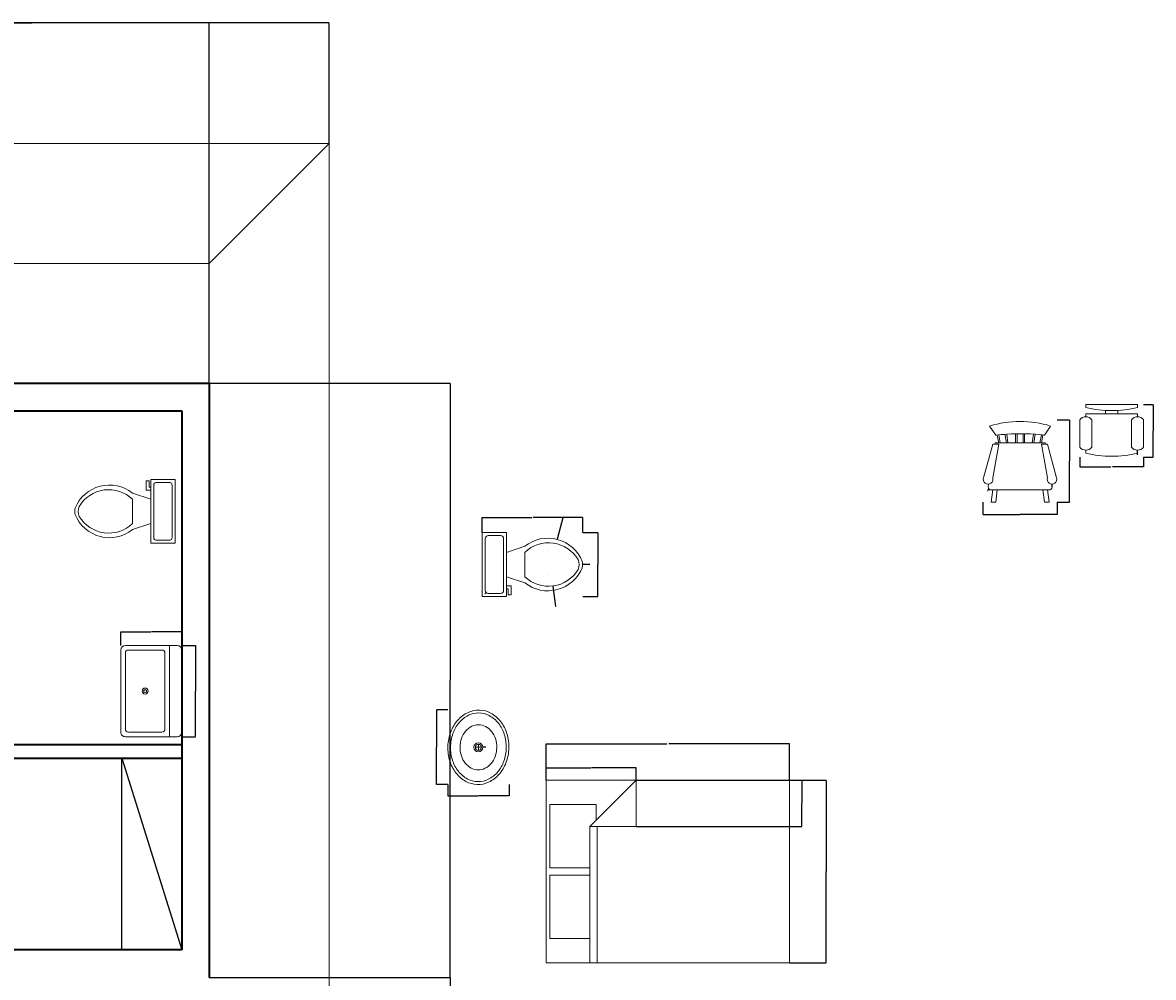
# Model space of a CAD drawing. Units: millimetres. Extents: x -8052 to 19968, y -37825 to -17505.
# Tile 10 of 10: x 10533 to 19968, y -25475 to -17505. Entities that reach past the tile are written whole.
import ezdxf

# ---------------------------------------------------------------- set-up
doc = ezdxf.new("R2010")
doc.units = ezdxf.units.MM
doc.header["$MEASUREMENT"] = 0
for name, color, linetype, lineweight in [('A-ANNO-DIMS', 2, 'Continuous', 18), ('A-FLOR', 8, 'Continuous', 18), ('A-FLOR-CASE', 9, 'Continuous', 25), ('A-FLOR-FIXT', 9, 'Continuous', 18), ('A-FURN', 8, 'Continuous', 18), ('A-WALL', 7, 'Continuous', 35)]:
    doc.layers.add(name, color=color, linetype=linetype, lineweight=lineweight)
doc.styles.get("Standard").update_dxf_attribs({"font": 'arial.ttf'})
doc.dimstyles.get("Standard").update_dxf_attribs({"dimtxt": 1.054, "dimasz": 1.055, "dimexe": 0.18, "dimexo": 0.0625, "dimgap": 0.09, "dimtad": 0, "dimtih": 1, "dimtoh": 1, "dimdec": 4, "dimzin": 0, "dimdsep": 46, "dimtxsty": 'Standard', "dimcen": 0.09, "dimadec": 0, "dimazin": 0, "dimtfac": 1, "dimtdec": 4, "dimtofl": 0, "dimtmove": 0, "dimatfit": 3, "dimfxl": 1, "dimtolj": 1, "dimtzin": 0, "dimarcsym": 0})

# ---------------------------------------------------------------- blocks, each defined once
blk = doc.blocks.new('Chair - Desk')
for p, q in [((-8.5, 0), (-8.5, -1)), ((-8.5, 0), (8.5, 0)), ((8.5, 0), (8.5, -1)), ((-8.5, -3), (-8.5, -4)), ((-8.5, -3), (8.5, -3)), ((-2, -3), (-2, -1.9355)), ((2, -1.9576), (2, -3)), ((8.5, -3), (8.5, -4)), ((-10.5, -5), (-10.5, -14)), ((-6.5, -14), (-6.5, -5)), ((6.5, -5), (6.5, -14)), ((10.5, -14), (10.5, -5)), ((-8.5, -15), (-8.5, -16)), ((8.5, -15), (8.5, -16))]:
    blk.add_line(p, q)
for centre, radius, start, end in [((0, 34.625), 36.625, 256.5803, 283.4197), ((-8.5, -6.5), 2.5, 36.8699, 143.1301), ((8.5, -6.5), 2.5, 36.8699, 143.1301), ((-8.5, -12.5), 2.5, 216.8699, 323.1301), ((8.5, -12.5), 2.5, 216.8699, 323.1301), ((0, 19.625), 36.625, 256.5803, 283.4197)]:
    blk.add_arc(centre, radius, start, end)
blk = doc.blocks.new('Chair - Rocking')
for p, q in [((-8, -4.5), (-10, -1.5)), ((8, -4.5), (10, -1.5)), ((-8.23428, -6.99939), (-8.3093, -7.47958)), ((-8.23041, -7), (8.23915, -7)), ((-7.5, -4.5), (-7, -7)), ((-6.5, -7), (-7.02225, -4.43)), ((-4.5, -7), (-4.96674, -4.19951)), ((-4, -7), (-4.40532, -4.16272)), ((-1.5, -4.05012), (-1.5, -7)), ((-1, -7), (-1, -4.05012)), ((1, -7), (1, -4.04655)), ((1.5, -4.05012), (1.5, -7)), ((4, -7), (4.40187, -4.18694)), ((4.5, -7), (4.96761, -4.19437)), ((6.5, -7), (7, -4.4057)), ((7.5, -4.5), (7, -7)), ((8.31071, -7.48854), (8.23449, -7.00073)), ((-9, -7.5), (-12, -18.49999)), ((-7, -7.5), (-9, -7.5)), ((-9, -18.49999), (-7, -7.5)), ((7, -7.5), (9, -7.5)), ((9, -18.49999), (7, -7.5)), ((9, -7.5), (12, -18.49999)), ((-10.36644, -20.64523), (-10.5, -21.49999)), ((10.5, -21.49999), (10.3575, -20.58798)), ((-9, -22.49999), (-9.5, -26.49999)), ((0, -22.49999), (-9.5, -22.49999)), ((-8, -26.49999), (-7.5, -22.49999)), ((0, -22.49999), (9.5, -22.49999)), ((8, -26.49999), (7.5, -22.49999)), ((9, -22.49999), (9.5, -26.49999)), ((-9.5, -26.49999), (-8, -26.49999)), ((9.5, -26.49999), (8, -26.49999))]:
    blk.add_line(p, q)
for centre, radius, start, end in [((0, -34.08333), 34.08333, 72.93847, 107.0615), ((0, -68.25004), 64.25, 93.92211, 97.15267), ((0, -68.25004), 64.25, 82.84733, 93.92211), ((-10.5, -18.99999), 1.58114, 161.5651, 18.43495), ((10.5, -18.99999), 1.58114, 161.5651, 18.43495), ((-9.5, -21.49999), 1, 180, 270), ((9.5, -21.49999), 1, 270, 0)]:
    blk.add_arc(centre, radius, start, end)
blk = doc.blocks.new('Toilet - top')
for p, q in [((9.5, -6), (9.5, -2)), ((-10, -8.5), (-8, -8.5)), ((-10, -9.5), (-10, -8.5)), ((-7, -9.5), (-10, -9.5)), ((-8, -8.5), (-8, -8)), ((-7, -8), (-7, -9.5)), ((-4, -8), (-6, -14)), ((4, -8), (6, -14)), ((4, -14), (-4, -14))]:
    blk.add_line(p, q)
blk.add_lwpolyline([(10.5, -8), (10.5, 0), (-10.5, 0), (-10.5, -8)], close=True)
for points in [[(-9.5, -2), (-9.5, -6)], [(8.5, -1), (-8.5, -1)], [(-8.5, -7), (8.5, -7)]]:
    blk.add_lwpolyline(points)
for centre, radius, start, end in [((-8.62, -1.88), 0.884, 81.8699, 188.1301), ((8.62, -1.88), 0.884, 351.8699, 98.1301), ((-8.62, -6.12), 0.884, 171.8699, 278.1301), ((8.62, -6.12), 0.884, 261.8699, 8.1301), ((3.52, -21.58), 12.17, 141.4691, 247.9714), ((4.2, -21.82), 11.33, 136.3677, 238.9468), ((-3.52, -21.58), 12.17, 292.0284, 38.5307), ((-4.2, -21.82), 11.33, 301.053, 43.6321), ((0, -27.88), 4, 245.7318, 294.2682), ((0, -29), 4, 254.8605, 285.1395)]:
    blk.add_arc(centre, radius, start, end)
blk = doc.blocks.new('Sink - Oval top')
for p, q in [((-1, 0), (1, 0)), ((0, 1), (0, -1))]:
    blk.add_line(p, q)
for points in [[(-12.23, 0.39, 0.117634), (-11.46, -3.36, 0.104469), (-8.88, -6.8, 0.090016), (-5.08, -9.07, 0.08192), (-0.32, -10.02, 0.08192), (4.49, -9.38, 0.090016), (8.42, -7.36, 0.104469), (11.22, -4.09, 0.117634), (12.23, -0.39, 0.117634), (11.46, 3.36, 0.104469), (8.88, 6.8, 0.090016), (5.08, 9.07, 0.08192), (0.32, 10.02, 0.08192), (-4.49, 9.38, 0.090016), (-8.42, 7.36, 0.104469), (-11.22, 4.09, 0.117634)], [(-11.29, 0.16, 0.118622), (-10.52, -3.25, 0.104678), (-8.07, -6.36, 0.089562), (-4.54, -8.37, 0.081185), (-0.13, -9.15, 0.081185), (4.3, -8.49, 0.089562), (7.89, -6.58, 0.104678), (10.42, -3.55, 0.118622), (11.29, -0.16, 0.118622), (10.52, 3.25, 0.104678), (8.07, 6.36, 0.089562), (4.54, 8.37, 0.081185), (0.13, 9.15, 0.081185), (-4.3, 8.49, 0.089562), (-7.89, 6.58, 0.104678), (-10.42, 3.55, 0.118622)], [(-7.42, 0.08, 0.118283), (-6.91, -2.17, 0.104607), (-5.29, -4.21, 0.089718), (-2.97, -5.53, 0.081436), (-0.07, -6.04, 0.081436), (2.84, -5.59, 0.089718), (5.2, -4.33, 0.104607), (6.86, -2.32, 0.118283), (7.42, -0.08, 0.118283), (6.91, 2.17, 0.104607), (5.29, 4.21, 0.089718), (2.97, 5.53, 0.081436), (0.07, 6.04, 0.081436), (-2.84, 5.59, 0.089718), (-5.2, 4.33, 0.104607), (-6.86, 2.32, 0.118283)]]:
    blk.add_lwpolyline(points, format="xyb", close=True)
for radius in [1.5, 1]:
    blk.add_circle((0, 0), radius)
blk = doc.blocks.new('Bed - Queen')
for p, q in [((0, -80.00003), (0, 0)), ((0, 0), (59.99999, 0)), ((59.99999, 0), (59.99999, -80.00003)), ((7.99999, -1.2), (28.79998, -1.2)), ((7.99999, -14.4), (7.99999, -1.2)), ((28.79998, -1.2), (28.79998, -14.4)), ((31.19999, -1.2), (51.99999, -1.2)), ((31.19999, -14.4), (31.19999, -1.2)), ((51.99999, -1.2), (51.99999, -16.4)), ((0, -14.4), (44.8, -14.4)), ((59.99999, -29.6), (44.8, -14.4)), ((44.8, -14.4), (44.8, -29.6)), ((44.8, -16.8), (0, -16.8)), ((51.99999, -16.4), (46.79936, -16.4)), ((44.8, -29.6), (59.99999, -29.6)), ((59.99999, -80.00003), (0, -80.00003))]:
    blk.add_line(p, q)
blk = doc.blocks.new('Sink-single - 30 in top')
blk.add_line((-15, -3.999996), (15, -3.999996))
for points in [[(-13.5, 0), (13.5, 0)], [(-15, -18.499996), (-15, -1.5)], [(15, -1.5), (15, -18.499996)], [(-13.5, -17.499996), (-13.5, -6.499996)], [(-12.5, -5.499996), (12.5, -5.499996)], [(13.5, -6.499996), (13.5, -17.499996)], [(12.5, -18.499996), (-12.5, -18.499996)], [(13.5, -19.999996), (-13.5, -19.999996)]]:
    blk.add_lwpolyline(points)
for radius in [1, 0.5]:
    blk.add_circle((0, -11.999996), radius)
for centre, radius, start, end in [((-13.5, -1.5), 1.5, 90, 180), ((13.5, -1.5), 1.5, 0, 90), ((-12.5, -6.499996), 1, 90, 180), ((12.5, -6.499996), 1, 0, 90), ((-13.5, -18.499996), 1.5, 180, 270), ((-12.5, -17.499996), 1, 180, 270), ((12.5, -17.499996), 1, 270, 0), ((13.5, -18.499996), 1.5, 270, 0)]:
    blk.add_arc(centre, radius, start, end)
blk = doc.blocks.new('CABINET-RECESSED-1600')
for p, q in [((500, 1600), (0, 0)), ((500, 0), (500, 1600))]:
    blk.add_line(p, q)
blk = doc.blocks.new('*D34')
at = {"layer": 'A-ANNO-DIMS', "color": 0, "lineweight": -2, "transparency": 16777216}
for p, q in [((14901.3, -23828.8), (14901.3, -23523.9)), ((14902.3, -23524.1), (15909.3, -23524.1)), ((16932.2, -23524.1), (15925.3, -23524.1)), ((16933.3, -23828.8), (16933.3, -23523.9))]:
    blk.add_line(p, q, dxfattribs=at)
at = {"layer": 'A-ANNO-DIMS', "color": 0, "lineweight": 100, "transparency": 16777216}
for points in [[(14902.3, -23523.9), (14902.3, -23524.2), (14901.3, -23524.1)], [(16932.2, -23523.9), (16932.2, -23524.2), (16933.3, -23524.1)]]:
    blk.add_solid(points, dxfattribs=at)
at = {"layer": 'Defpoints', "color": 0, "lineweight": 100, "transparency": 16777216}
for p in [(14901.3, -23524.1), (14901.3, -23828.9), (16933.3, -23828.9)]:
    blk.add_point(p, dxfattribs=at)
at = {"layer": 'A-ANNO-DIMS', "color": 0, "transparency": 16777216, "insert": (15917.3, -23524.1), "char_height": 1.054, "attachment_point": 5}
blk.add_mtext('\\A1;QUEEN BED 2032 TYP.', dxfattribs=at)
blk = doc.blocks.new('*D35')
at = {"layer": 'A-ANNO-DIMS', "color": 0, "lineweight": -2, "transparency": 16777216}
for p, q in [((16933.3, -23828.9), (17238.3, -23828.9)), ((17238.1, -23829.9), (17238.1, -24590.2)), ((17238.1, -25351.8), (17238.1, -24591.5)), ((16933.3, -25352.9), (17238.3, -25352.9))]:
    blk.add_line(p, q, dxfattribs=at)
at = {"layer": 'A-ANNO-DIMS', "color": 0, "lineweight": 100, "transparency": 16777216}
for points in [[(17237.9, -23829.9), (17238.2, -23829.9), (17238.1, -23828.9)], [(17237.9, -25351.8), (17238.2, -25351.8), (17238.1, -25352.9)]]:
    blk.add_solid(points, dxfattribs=at)
at = {"layer": 'Defpoints', "color": 0, "lineweight": 100, "transparency": 16777216}
for p in [(16933.3, -23828.9), (17238.1, -23828.9), (16933.3, -25352.9)]:
    blk.add_point(p, dxfattribs=at)
at = {"layer": 'A-ANNO-DIMS', "color": 0, "transparency": 16777216, "insert": (17238.1, -24590.9), "char_height": 1.054, "attachment_point": 5}
blk.add_mtext('\\A1;1524 TYP.', dxfattribs=at)
blk = doc.blocks.new('*D36')
at = {"layer": 'A-ANNO-DIMS', "color": 0, "lineweight": -2, "transparency": 16777216}
for p, q in [((14367.7, -21761.6), (14367.7, -21635.5)), ((14368.7, -21635.7), (14782.8, -21635.7)), ((15206, -21635.7), (14791.9, -21635.7)), ((15207, -21761.6), (15207, -21635.5))]:
    blk.add_line(p, q, dxfattribs=at)
at = {"layer": 'A-ANNO-DIMS', "color": 0, "lineweight": 100, "transparency": 16777216}
for points in [[(14368.7, -21635.6), (14368.7, -21635.9), (14367.7, -21635.7)], [(15206, -21635.6), (15206, -21635.9), (15207, -21635.7)]]:
    blk.add_solid(points, dxfattribs=at)
at = {"layer": 'Defpoints', "color": 0, "lineweight": 100, "transparency": 16777216}
for p in [(14367.7, -21635.7), (14367.7, -21761.6), (15207, -21761.6)]:
    blk.add_point(p, dxfattribs=at)
at = {"layer": 'A-ANNO-DIMS', "color": 0, "transparency": 16777216, "insert": (14787.3, -21635.7), "char_height": 1.054, "attachment_point": 5}
blk.add_mtext('\\A1;WC 839 TYP.', dxfattribs=at)
blk = doc.blocks.new('*D37')
at = {"layer": 'A-ANNO-DIMS', "color": 0, "lineweight": -2, "transparency": 16777216}
for p, q in [((15207.1, -21761.6), (15333.1, -21761.6)), ((15332.9, -21762.7), (15332.9, -22027.7)), ((15332.9, -22294), (15332.9, -22029)), ((15207.1, -22295), (15333.1, -22295))]:
    blk.add_line(p, q, dxfattribs=at)
at = {"layer": 'A-ANNO-DIMS', "color": 0, "lineweight": 100, "transparency": 16777216}
for points in [[(15332.8, -21762.7), (15333.1, -21762.7), (15332.9, -21761.6)], [(15332.8, -22294), (15333.1, -22294), (15332.9, -22295)]]:
    blk.add_solid(points, dxfattribs=at)
at = {"layer": 'Defpoints', "color": 0, "lineweight": 100, "transparency": 16777216}
for p in [(15207, -21761.6), (15332.9, -21761.6), (15207, -22295)]:
    blk.add_point(p, dxfattribs=at)
at = {"layer": 'A-ANNO-DIMS', "color": 0, "transparency": 16777216, "insert": (15332.9, -22028.3), "char_height": 1.054, "attachment_point": 5}
blk.add_mtext('\\A1;533 TYP.', dxfattribs=at)
blk = doc.blocks.new('*D38')
at = {"layer": 'A-ANNO-DIMS', "color": 0, "lineweight": -2, "transparency": 16777216}
for p, q in [((14080.1, -23242.4), (13986.4, -23242.4)), ((13986.6, -23243.4), (13986.6, -23553.5)), ((13986.6, -23864.9), (13986.6, -23554.8)), ((14080.1, -23865.9), (13986.4, -23865.9))]:
    blk.add_line(p, q, dxfattribs=at)
at = {"layer": 'A-ANNO-DIMS', "color": 0, "lineweight": 100, "transparency": 16777216}
for points in [[(13986.4, -23243.4), (13986.8, -23243.4), (13986.6, -23242.4)], [(13986.4, -23864.9), (13986.8, -23864.9), (13986.6, -23865.9)]]:
    blk.add_solid(points, dxfattribs=at)
at = {"layer": 'Defpoints', "color": 0, "lineweight": 100, "transparency": 16777216}
for p in [(14080.1, -23242.4), (13986.6, -23865.9), (14080.1, -23865.9)]:
    blk.add_point(p, dxfattribs=at)
at = {"layer": 'A-ANNO-DIMS', "color": 0, "transparency": 16777216, "insert": (13986.6, -23554.2), "char_height": 1.054, "attachment_point": 5}
blk.add_mtext('\\A1;BASIN 624 TYP.', dxfattribs=at)
blk = doc.blocks.new('*D39')
at = {"layer": 'A-ANNO-DIMS', "color": 0, "lineweight": -2, "transparency": 16777216}
for p, q in [((14080.1, -23866), (14080.1, -23959.7)), ((14591.6, -23866), (14591.6, -23959.7)), ((14081.2, -23959.5), (14332.8, -23959.5)), ((14590.5, -23959.5), (14338.9, -23959.5))]:
    blk.add_line(p, q, dxfattribs=at)
at = {"layer": 'A-ANNO-DIMS', "color": 0, "lineweight": 100, "transparency": 16777216}
for points in [[(14081.2, -23959.3), (14081.2, -23959.7), (14080.1, -23959.5)], [(14590.5, -23959.3), (14590.5, -23959.7), (14591.6, -23959.5)]]:
    blk.add_solid(points, dxfattribs=at)
at = {"layer": 'Defpoints', "color": 0, "lineweight": 100, "transparency": 16777216}
for p in [(14080.1, -23865.9), (14591.6, -23865.9), (14591.6, -23959.5)]:
    blk.add_point(p, dxfattribs=at)
at = {"layer": 'A-ANNO-DIMS', "color": 0, "transparency": 16777216, "insert": (14335.9, -23959.5), "char_height": 1.054, "attachment_point": 5}
blk.add_mtext('\\A1;511 TYP.', dxfattribs=at)
blk = doc.blocks.new('*D40')
at = {"layer": 'A-ANNO-DIMS', "color": 0, "lineweight": -2, "transparency": 16777216}
for p, q in [((19353.6, -21133.4), (19353.6, -21213.5)), ((19887, -21133.4), (19887, -21213.5)), ((19354.7, -21213.3), (19614.4, -21213.3)), ((19886, -21213.3), (19626.3, -21213.3))]:
    blk.add_line(p, q, dxfattribs=at)
at = {"layer": 'A-ANNO-DIMS', "color": 0, "lineweight": 100, "transparency": 16777216}
for points in [[(19354.7, -21213.1), (19354.7, -21213.5), (19353.6, -21213.3)], [(19886, -21213.1), (19886, -21213.5), (19887, -21213.3)]]:
    blk.add_solid(points, dxfattribs=at)
at = {"layer": 'Defpoints', "color": 0, "lineweight": 100, "transparency": 16777216}
for p in [(19353.6, -21133.3), (19887, -21133.3), (19887, -21213.3)]:
    blk.add_point(p, dxfattribs=at)
at = {"layer": 'A-ANNO-DIMS', "color": 0, "transparency": 16777216, "insert": (19620.3, -21213.3), "char_height": 1.054, "attachment_point": 5}
blk.add_mtext('\\A1;DESK CHAIR 533', dxfattribs=at)
blk = doc.blocks.new('*D41')
at = {"layer": 'A-ANNO-DIMS', "color": 0, "lineweight": -2, "transparency": 16777216}
for p, q in [((19887.1, -20693), (19967.2, -20693)), ((19967, -20694.1), (19967, -20912.5)), ((19967, -21132.2), (19967, -20913.8)), ((19887.1, -21133.3), (19967.2, -21133.3))]:
    blk.add_line(p, q, dxfattribs=at)
at = {"layer": 'A-ANNO-DIMS', "color": 0, "lineweight": 100, "transparency": 16777216}
for points in [[(19966.9, -20694.1), (19967.2, -20694.1), (19967, -20693)], [(19966.9, -21132.2), (19967.2, -21132.2), (19967, -21133.3)]]:
    blk.add_solid(points, dxfattribs=at)
at = {"layer": 'Defpoints', "color": 0, "lineweight": 100, "transparency": 16777216}
for p in [(19887, -20693), (19967, -20693), (19887, -21133.3)]:
    blk.add_point(p, dxfattribs=at)
at = {"layer": 'A-ANNO-DIMS', "color": 0, "transparency": 16777216, "insert": (19967, -20913.2), "char_height": 1.05, "attachment_point": 5}
blk.add_mtext('\\A1;440', dxfattribs=at)
blk = doc.blocks.new('*D42')
at = {"layer": 'A-ANNO-DIMS', "color": 0, "lineweight": -2, "transparency": 16777216}
for p, q in [((19166.6, -20821.7), (19269.6, -20821.7)), ((19269.4, -20822.8), (19269.4, -21164)), ((19269.4, -21506.5), (19269.4, -21165.3)), ((19166.6, -21507.5), (19269.6, -21507.5))]:
    blk.add_line(p, q, dxfattribs=at)
at = {"layer": 'A-ANNO-DIMS', "color": 0, "lineweight": 100, "transparency": 16777216}
for points in [[(19269.2, -20822.8), (19269.6, -20822.8), (19269.4, -20821.7)], [(19269.2, -21506.5), (19269.6, -21506.5), (19269.4, -21507.5)]]:
    blk.add_solid(points, dxfattribs=at)
at = {"layer": 'Defpoints', "color": 0, "lineweight": 100, "transparency": 16777216}
for p in [(19166.5, -20821.7), (19269.4, -20821.7), (19166.5, -21507.5)]:
    blk.add_point(p, dxfattribs=at)
at = {"layer": 'A-ANNO-DIMS', "color": 0, "transparency": 16777216, "insert": (19269.4, -21164.6), "char_height": 1.054, "attachment_point": 5}
blk.add_mtext('\\A1;ROCKER 686', dxfattribs=at)
blk = doc.blocks.new('*D43')
at = {"layer": 'A-ANNO-DIMS', "color": 0, "lineweight": -2, "transparency": 16777216}
for p, q in [((18545.9, -21507.6), (18545.9, -21610.6)), ((19166.5, -21507.6), (19166.5, -21610.6)), ((18546.9, -21610.4), (18855.1, -21610.4)), ((19165.5, -21610.4), (18857.4, -21610.4))]:
    blk.add_line(p, q, dxfattribs=at)
at = {"layer": 'A-ANNO-DIMS', "color": 0, "lineweight": 100, "transparency": 16777216}
for points in [[(18546.9, -21610.2), (18546.9, -21610.6), (18545.9, -21610.4)], [(19165.5, -21610.2), (19165.5, -21610.6), (19166.5, -21610.4)]]:
    blk.add_solid(points, dxfattribs=at)
at = {"layer": 'Defpoints', "color": 0, "lineweight": 100, "transparency": 16777216}
for p in [(18545.9, -21507.5), (19166.5, -21507.5), (19166.5, -21610.4)]:
    blk.add_point(p, dxfattribs=at)
at = {"layer": 'A-ANNO-DIMS', "color": 0, "transparency": 16777216, "insert": (18856.2, -21610.4), "char_height": 1.05, "attachment_point": 5}
blk.add_mtext('\\A1;621', dxfattribs=at)
blk = doc.blocks.new('*D44')
at = {"layer": 'A-ANNO-DIMS', "color": 0, "lineweight": -2, "transparency": 16777216}
for p, q in [((11860, -22703.8), (11974.5, -22703.8)), ((11974.3, -22704.9), (11974.3, -23084.2)), ((11974.3, -23464.7), (11974.3, -23085.4)), ((11860, -23465.8), (11974.5, -23465.8))]:
    blk.add_line(p, q, dxfattribs=at)
at = {"layer": 'A-ANNO-DIMS', "color": 0, "lineweight": 100, "transparency": 16777216}
for points in [[(11974.1, -22704.9), (11974.5, -22704.9), (11974.3, -22703.8)], [(11974.1, -23464.7), (11974.5, -23464.7), (11974.3, -23465.8)]]:
    blk.add_solid(points, dxfattribs=at)
at = {"layer": 'Defpoints', "color": 0, "lineweight": 100, "transparency": 16777216}
for p in [(11860, -22703.8), (11860, -23465.8), (11974.3, -23465.8)]:
    blk.add_point(p, dxfattribs=at)
at = {"layer": 'A-ANNO-DIMS', "color": 0, "transparency": 16777216, "insert": (11974.3, -23084.8), "char_height": 1.054, "attachment_point": 5}
blk.add_mtext('\\A1;VANITY SINK 762 TYP.', dxfattribs=at)
blk = doc.blocks.new('*D45')
at = {"layer": 'A-ANNO-DIMS', "color": 0, "lineweight": -2, "transparency": 16777216}
for p, q in [((11352, -22703.7), (11352, -22589.3)), ((11353, -22589.5), (11602.9, -22589.5)), ((11858.9, -22589.5), (11609, -22589.5)), ((11860, -22703.7), (11860, -22589.3))]:
    blk.add_line(p, q, dxfattribs=at)
at = {"layer": 'A-ANNO-DIMS', "color": 0, "lineweight": 100, "transparency": 16777216}
for points in [[(11353, -22589.3), (11353, -22589.7), (11352, -22589.5)], [(11858.9, -22589.3), (11858.9, -22589.7), (11860, -22589.5)]]:
    blk.add_solid(points, dxfattribs=at)
at = {"layer": 'Defpoints', "color": 0, "lineweight": 100, "transparency": 16777216}
for p in [(11860, -22589.5), (11352, -22703.8), (11860, -22703.8)]:
    blk.add_point(p, dxfattribs=at)
at = {"layer": 'A-ANNO-DIMS', "color": 0, "transparency": 16777216, "insert": (11606, -22589.5), "char_height": 1.054, "attachment_point": 5}
blk.add_mtext('\\A1;508 TYP.', dxfattribs=at)
blk = doc.blocks.new('*D84')
at = {"layer": 'A-ANNO-DIMS', "color": 0, "lineweight": -2, "transparency": 16777216}
for p, q in [((-7040, -18514.8), (-7040, -17505.2)), ((-7039, -17505.3), (3022.9, -17505.3)), ((13088.9, -17505.3), (3027.1, -17505.3)), ((13090, -18514.8), (13090, -17505.2))]:
    blk.add_line(p, q, dxfattribs=at)
at = {"layer": 'A-ANNO-DIMS', "color": 0, "lineweight": 100, "transparency": 16777216}
for points in [[(-7039, -17505.2), (-7039, -17505.5), (-7040, -17505.3)], [(13088.9, -17505.2), (13088.9, -17505.5), (13090, -17505.3)]]:
    blk.add_solid(points, dxfattribs=at)
at = {"layer": 'Defpoints', "color": 0, "lineweight": 100, "transparency": 16777216}
for p in [(13090, -17505.3), (-7040, -18514.8), (13090, -18514.8)]:
    blk.add_point(p, dxfattribs=at)
at = {"layer": 'A-ANNO-DIMS', "color": 0, "transparency": 16777216, "insert": (3025, -17505.3), "char_height": 1.05, "attachment_point": 5}
blk.add_mtext('\\A1;20130', dxfattribs=at)
blk = doc.blocks.new('*D93')
at = {"layer": 'A-ANNO-DIMS', "color": 0, "lineweight": -2, "transparency": 16777216}
for p, q in [((9130, -20514.8), (9130, -17505.2)), ((9131, -17505.3), (10608.3, -17505.3)), ((12088.9, -17505.3), (10611.7, -17505.3)), ((12090, -20514.8), (12090, -17505.2))]:
    blk.add_line(p, q, dxfattribs=at)
at = {"layer": 'A-ANNO-DIMS', "color": 0, "lineweight": 100, "transparency": 16777216}
for points in [[(9131, -17505.2), (9131, -17505.5), (9130, -17505.3)], [(12088.9, -17505.2), (12088.9, -17505.5), (12090, -17505.3)]]:
    blk.add_solid(points, dxfattribs=at)
at = {"layer": 'Defpoints', "color": 0, "lineweight": 100, "transparency": 16777216}
for p in [(12090, -17505.3), (9130, -20514.8), (12090, -20514.8)]:
    blk.add_point(p, dxfattribs=at)
at = {"layer": 'A-ANNO-DIMS', "color": 0, "transparency": 16777216, "insert": (10610, -17505.3), "char_height": 1.05, "attachment_point": 5}
blk.add_mtext('\\A1;2960', dxfattribs=at)
blk = doc.blocks.new('*D96')
at = {"layer": 'A-ANNO-DIMS', "color": 0, "lineweight": -2, "transparency": 16777216}
for p, q in [((12090, -20514.8), (14099.7, -20514.8)), ((14099.5, -20515.9), (14099.5, -22994.2)), ((14099.5, -25473.8), (14099.5, -22995.5)), ((12090, -25474.8), (14099.7, -25474.8))]:
    blk.add_line(p, q, dxfattribs=at)
at = {"layer": 'A-ANNO-DIMS', "color": 0, "lineweight": 100, "transparency": 16777216}
for points in [[(14099.3, -20515.9), (14099.7, -20515.9), (14099.5, -20514.8)], [(14099.3, -25473.8), (14099.7, -25473.8), (14099.5, -25474.8)]]:
    blk.add_solid(points, dxfattribs=at)
at = {"layer": 'Defpoints', "color": 0, "lineweight": 100, "transparency": 16777216}
for p in [(12090, -20514.8), (12090, -25474.8), (14099.5, -25474.8)]:
    blk.add_point(p, dxfattribs=at)
at = {"layer": 'A-ANNO-DIMS', "color": 0, "transparency": 16777216, "insert": (14099.5, -22994.8), "char_height": 1.05, "attachment_point": 5}
blk.add_mtext('\\A1;4960', dxfattribs=at)
blk = doc.blocks.new('*D97')
at = {"layer": 'A-ANNO-DIMS', "color": 0, "lineweight": -2, "transparency": 16777216}
for p, q in [((12090, -25474.8), (14099.7, -25474.8)), ((14099.5, -25475.9), (14099.5, -27724.2)), ((14099.5, -29973.8), (14099.5, -27725.5)), ((10410, -29974.8), (14099.7, -29974.8))]:
    blk.add_line(p, q, dxfattribs=at)
at = {"layer": 'A-ANNO-DIMS', "color": 0, "lineweight": 100, "transparency": 16777216}
for points in [[(14099.3, -25475.9), (14099.7, -25475.9), (14099.5, -25474.8)], [(14099.3, -29973.8), (14099.7, -29973.8), (14099.5, -29974.8)]]:
    blk.add_solid(points, dxfattribs=at)
at = {"layer": 'Defpoints', "color": 0, "lineweight": 100, "transparency": 16777216}
for p in [(12090, -25474.8), (10410, -29974.8), (14099.5, -29974.8)]:
    blk.add_point(p, dxfattribs=at)
at = {"layer": 'A-ANNO-DIMS', "color": 0, "transparency": 16777216, "insert": (14099.5, -27724.8), "char_height": 1.05, "attachment_point": 5}
blk.add_mtext('\\A1;4500', dxfattribs=at)
blk = doc.blocks.new('*D123')
at = {"layer": 'A-ANNO-DIMS', "color": 0, "lineweight": -2, "transparency": 16777216}
for p, q in [((7260, -25474.8), (7260, -17505.2)), ((7261, -17505.3), (9673.3, -17505.3)), ((12088.9, -17505.3), (9676.7, -17505.3)), ((12090, -25474.8), (12090, -17505.2))]:
    blk.add_line(p, q, dxfattribs=at)
at = {"layer": 'A-ANNO-DIMS', "color": 0, "lineweight": 100, "transparency": 16777216}
for points in [[(7261, -17505.2), (7261, -17505.5), (7260, -17505.3)], [(12088.9, -17505.2), (12088.9, -17505.5), (12090, -17505.3)]]:
    blk.add_solid(points, dxfattribs=at)
at = {"layer": 'Defpoints', "color": 0, "lineweight": 100, "transparency": 16777216}
for p in [(7260, -17505.3), (7260, -25474.8), (12090, -25474.8)]:
    blk.add_point(p, dxfattribs=at)
at = {"layer": 'A-ANNO-DIMS', "color": 0, "transparency": 16777216, "insert": (9675, -17505.3), "char_height": 1.05, "attachment_point": 5}
blk.add_mtext('\\A1;4830', dxfattribs=at)
blk = doc.blocks.new('*D129')
at = {"layer": 'A-ANNO-DIMS', "color": 0, "lineweight": -2, "transparency": 16777216}
for p, q in [((14901.3, -23828.8), (14901.3, -23725.9)), ((14902.3, -23726.1), (15275.3, -23726.1)), ((15652.1, -23726.1), (15279.1, -23726.1)), ((15653.1, -23828.8), (15653.1, -23725.9))]:
    blk.add_line(p, q, dxfattribs=at)
at = {"layer": 'A-ANNO-DIMS', "color": 0, "lineweight": 100, "transparency": 16777216}
for points in [[(14902.3, -23725.9), (14902.3, -23726.3), (14901.3, -23726.1)], [(15652.1, -23725.9), (15652.1, -23726.3), (15653.1, -23726.1)]]:
    blk.add_solid(points, dxfattribs=at)
at = {"layer": 'Defpoints', "color": 0, "lineweight": 100, "transparency": 16777216}
for p in [(15653.1, -23726.1), (14901.3, -23828.9), (15653.1, -23828.9)]:
    blk.add_point(p, dxfattribs=at)
at = {"layer": 'A-ANNO-DIMS', "color": 0, "transparency": 16777216, "insert": (15277.2, -23726.1), "char_height": 1.05, "attachment_point": 5}
blk.add_mtext('\\A1;751.8', dxfattribs=at)
blk = doc.blocks.new('*D130')
at = {"layer": 'A-ANNO-DIMS', "color": 0, "lineweight": -2, "transparency": 16777216}
for p, q in [((15653.2, -23828.9), (17036.2, -23828.9)), ((17036, -23829.9), (17036, -24021.3)), ((17036, -24213.9), (17036, -24022.5)), ((15653.2, -24214.9), (17036.2, -24214.9))]:
    blk.add_line(p, q, dxfattribs=at)
at = {"layer": 'A-ANNO-DIMS', "color": 0, "lineweight": 100, "transparency": 16777216}
for points in [[(17035.8, -23829.9), (17036.2, -23829.9), (17036, -23828.9)], [(17035.8, -24213.9), (17036.2, -24213.9), (17036, -24214.9)]]:
    blk.add_solid(points, dxfattribs=at)
at = {"layer": 'Defpoints', "color": 0, "lineweight": 100, "transparency": 16777216}
for p in [(15653.1, -23828.9), (15653.1, -24214.9), (17036, -24214.9)]:
    blk.add_point(p, dxfattribs=at)
at = {"layer": 'A-ANNO-DIMS', "color": 0, "transparency": 16777216, "insert": (17036, -24021.9), "char_height": 1.05, "attachment_point": 5}
blk.add_mtext('\\A1;386.1', dxfattribs=at)
blk = doc.blocks.new('*D137')
at = {"layer": 'A-ANNO-DIMS', "color": 0, "lineweight": -2, "transparency": 16777216}
for p, q in [((15041.5, -21639.4), (14994.6, -21817.8)), ((15042.5, -21639.4), (15041.5, -21639.4)), ((14915.7, -22117.7), (14915.9, -22117.7)), ((14915.8, -22117.8), (14915.8, -22117.6))]:
    blk.add_line(p, q, dxfattribs=at)
at = {"layer": 'A-ANNO-DIMS', "color": 0, "lineweight": 100, "transparency": 16777216}
blk.add_solid([(14994.4, -21817.7), (14994.8, -21817.8), (14994.3, -21818.8)], dxfattribs=at)
at = {"layer": 'Defpoints', "color": 0, "lineweight": 100, "transparency": 16777216}
for p in [(14994.3, -21818.8), (14915.8, -22117.7)]:
    blk.add_point(p, dxfattribs=at)
at = {"layer": 'A-ANNO-DIMS', "color": 0, "transparency": 16777216, "insert": (15045.9, -21639.4), "char_height": 1.054, "attachment_point": 5}
blk.add_mtext('\\A1;2X R309.1', dxfattribs=at)
blk = doc.blocks.new('*D138')
at = {"layer": 'A-ANNO-DIMS', "color": 0, "lineweight": -2, "transparency": 16777216}
for p, q in [((14921.7, -21921.7), (14921.9, -21921.7)), ((14921.8, -21921.7), (14921.8, -21921.6)), ((14983.2, -22378), (14960.3, -22207.9)), ((14984.2, -22378), (14983.2, -22378))]:
    blk.add_line(p, q, dxfattribs=at)
at = {"layer": 'A-ANNO-DIMS', "color": 0, "lineweight": 100, "transparency": 16777216}
blk.add_solid([(14960.5, -22207.9), (14960.1, -22207.9), (14960.2, -22206.9)], dxfattribs=at)
at = {"layer": 'Defpoints', "color": 0, "lineweight": 100, "transparency": 16777216}
for p in [(14921.8, -21921.7), (14960.2, -22206.9)]:
    blk.add_point(p, dxfattribs=at)
at = {"layer": 'A-ANNO-DIMS', "color": 0, "transparency": 16777216, "insert": (14988.2, -22378), "char_height": 1.054, "attachment_point": 5}
blk.add_mtext('\\A1;2X R287.76', dxfattribs=at)
blk = doc.blocks.new('*D139')
at = {"layer": 'A-ANNO-DIMS', "color": 0, "lineweight": -2, "transparency": 16777216}
for p, q in [((15104.2, -22028.3), (15104.3, -22028.3)), ((15104.3, -22028.4), (15104.3, -22028.2)), ((15266.8, -22028.3), (15206.9, -22028.3))]:
    blk.add_line(p, q, dxfattribs=at)
at = {"layer": 'A-ANNO-DIMS', "color": 0, "lineweight": 100, "transparency": 16777216}
blk.add_solid([(15206.9, -22028.2), (15206.9, -22028.5), (15205.9, -22028.3)], dxfattribs=at)
at = {"layer": 'Defpoints', "color": 0, "lineweight": 100, "transparency": 16777216}
for p in [(15104.3, -22028.3), (15205.9, -22028.3)]:
    blk.add_point(p, dxfattribs=at)
at = {"layer": 'A-ANNO-DIMS', "color": 0, "transparency": 16777216, "insert": (15270.3, -22028.3), "char_height": 1.054, "attachment_point": 5}
blk.add_mtext('\\A1;2X R101.6', dxfattribs=at)
blk = doc.blocks.new('*D140')
at = {"layer": 'A-ANNO-DIMS', "color": 0, "lineweight": -2, "transparency": 16777216}
for p, q in [((14389.9, -22272.8), (14398.7, -22264)), ((14415.2, -22247.4), (14415.4, -22247.4)), ((14415.3, -22247.5), (14415.3, -22247.3)), ((14388.8, -22272.8), (14389.9, -22272.8))]:
    blk.add_line(p, q, dxfattribs=at)
at = {"layer": 'A-ANNO-DIMS', "color": 0, "lineweight": 100, "transparency": 16777216}
blk.add_solid([(14398.5, -22263.9), (14398.8, -22264.2), (14399.4, -22263.3)], dxfattribs=at)
at = {"layer": 'Defpoints', "color": 0, "lineweight": 100, "transparency": 16777216}
for p in [(14399.4, -22263.3), (14415.3, -22247.4)]:
    blk.add_point(p, dxfattribs=at)
at = {"layer": 'A-ANNO-DIMS', "color": 0, "transparency": 16777216, "insert": (14385.3, -22272.8), "char_height": 1.054, "attachment_point": 5}
blk.add_mtext('\\A1;4X R22.45', dxfattribs=at)
blk = doc.blocks.new('*D141')
at = {"layer": 'A-ANNO-DIMS', "color": 0, "lineweight": -2, "transparency": 16777216}
for p, q in [((14335.8, -23554.2), (14335.9, -23554.2)), ((14335.9, -23554.2), (14335.9, -23554.1)), ((14396.8, -23554.2), (14375, -23554.2))]:
    blk.add_line(p, q, dxfattribs=at)
at = {"layer": 'A-ANNO-DIMS', "color": 0, "lineweight": 100, "transparency": 16777216}
blk.add_solid([(14375, -23554), (14375, -23554.3), (14374, -23554.2)], dxfattribs=at)
at = {"layer": 'Defpoints', "color": 0, "lineweight": 100, "transparency": 16777216}
for p in [(14297.8, -23554.2), (14374, -23554.2)]:
    blk.add_point(p, dxfattribs=at)
at = {"layer": 'A-ANNO-DIMS', "color": 0, "transparency": 16777216, "insert": (14398.8, -23554.2), "char_height": 1.05, "attachment_point": 5}
blk.add_mtext('\\A1;∅76.2', dxfattribs=at)
blk = doc.blocks.new('*D142')
at = {"layer": 'A-ANNO-DIMS', "color": 0, "lineweight": -2, "transparency": 16777216}
for p, q in [((19122.8, -21317), (19123, -21317)), ((19122.9, -21317.1), (19122.9, -21317)), ((19122.9, -21381.3), (19122.9, -21358.3)), ((19124, -21381.3), (19122.9, -21381.3))]:
    blk.add_line(p, q, dxfattribs=at)
at = {"layer": 'A-ANNO-DIMS', "color": 0, "lineweight": 100, "transparency": 16777216}
blk.add_solid([(19123.1, -21358.3), (19122.7, -21358.3), (19122.9, -21357.2)], dxfattribs=at)
at = {"layer": 'Defpoints', "color": 0, "lineweight": 100, "transparency": 16777216}
for p in [(19122.9, -21317), (19122.9, -21357.2)]:
    blk.add_point(p, dxfattribs=at)
at = {"layer": 'A-ANNO-DIMS', "color": 0, "transparency": 16777216, "insert": (19127.5, -21381.3), "char_height": 1.054, "attachment_point": 5}
blk.add_mtext('\\A1;2X R40.16', dxfattribs=at)
blk = doc.blocks.new('*D143')
at = {"layer": 'A-ANNO-DIMS', "color": 0, "lineweight": -2, "transparency": 16777216}
for p, q in [((18585.1, -21409.3), (18586.2, -21409.3)), ((18586.2, -21409.3), (18596.2, -21399.3)), ((18614.8, -21380.5), (18615, -21380.5)), ((18614.9, -21380.6), (18614.9, -21380.5))]:
    blk.add_line(p, q, dxfattribs=at)
at = {"layer": 'A-ANNO-DIMS', "color": 0, "lineweight": 100, "transparency": 16777216}
blk.add_solid([(18596.1, -21399.1), (18596.3, -21399.4), (18597, -21398.5)], dxfattribs=at)
at = {"layer": 'Defpoints', "color": 0, "lineweight": 100, "transparency": 16777216}
for p in [(18597, -21398.5), (18614.9, -21380.5)]:
    blk.add_point(p, dxfattribs=at)
at = {"layer": 'A-ANNO-DIMS', "color": 0, "transparency": 16777216, "insert": (18582, -21409.3), "char_height": 1.054, "attachment_point": 5}
blk.add_mtext('\\A1;2X R25.4', dxfattribs=at)
blk = doc.blocks.new('*D144')
at = {"layer": 'A-ANNO-DIMS', "color": 0, "lineweight": -2, "transparency": 16777216}
for p, q in [((19836.1, -21010.5), (19836.3, -21010.5)), ((19836.2, -21010.6), (19836.2, -21010.4)), ((19835.2, -21112.1), (19836.2, -21112.1)), ((19836.2, -21112.1), (19836.2, -21075.1))]:
    blk.add_line(p, q, dxfattribs=at)
at = {"layer": 'A-ANNO-DIMS', "color": 0, "lineweight": 100, "transparency": 16777216}
blk.add_solid([(19836.1, -21075.1), (19836.4, -21075.1), (19836.2, -21074)], dxfattribs=at)
at = {"layer": 'Defpoints', "color": 0, "lineweight": 100, "transparency": 16777216}
for p in [(19836.2, -21010.5), (19836.2, -21074)]:
    blk.add_point(p, dxfattribs=at)
at = {"layer": 'A-ANNO-DIMS', "color": 0, "transparency": 16777216, "insert": (19832.1, -21112.1), "char_height": 1.054, "attachment_point": 5}
blk.add_mtext('\\A1;4X R63.5', dxfattribs=at)

msp = doc.modelspace()

# ---------------------------------------------------------------- linework, layer by layer
at = {"layer": 'A-FLOR'}
for p, q in [((-4810.021, -18514.843), (13089.979, -18514.843)), ((12089.979, -19514.843), (13089.979, -18514.843)), ((13089.979, -18514.843), (13089.979, -26474.843)), ((-6040.021, -19514.843), (12089.979, -19514.843)), ((12089.979, -19514.843), (12089.979, -20514.843))]:
    msp.add_line(p, q, dxfattribs=at)
at = {"layer": 'A-WALL'}
for p, q in [((9359.979, -20514.843), (11859.979, -20514.843)), ((11859.979, -20514.843), (12089.979, -20514.843)), ((12089.979, -20514.843), (12089.979, -20744.843)), ((9359.979, -20744.843), (11859.979, -20744.843)), ((11859.979, -20744.843), (11859.979, -25244.843)), ((12089.979, -20744.843), (12089.979, -25244.843)), ((10209.02, -23529.843), (11859.979, -23529.843)), ((10209.02, -23644.843), (11859.979, -23644.843)), ((11859.979, -25244.843), (9359.979, -25244.843)), ((12089.979, -25244.843), (12089.979, -25474.843))]:
    msp.add_line(p, q, dxfattribs=at)

# ---------------------------------------------------------------- block references
at = {"layer": 'A-FLOR-CASE', "extrusion": (0, 0, -1), "zscale": -1}
msp.add_blockref('CABINET-RECESSED-1600', (-11859.98, -25244.843), dxfattribs=at)
at = {"layer": 'A-FLOR-FIXT', "xscale": 25.4, "yscale": 25.4, "zscale": 25.4}
for name, p, rotation in [('Toilet - top', (11805.594, -21584.722), 269.9999999999988), ('Toilet - top', (14367.66, -22028.334), 90), ('Sink-single - 30 in top', (11859.979, -23084.801), 270), ('Sink - Oval top', (14335.856, -23554.153), 270)]:
    msp.add_blockref(name, p, dxfattribs=dict(at, rotation=rotation))
at = {"layer": 'A-FURN', "xscale": 25.4, "yscale": 25.4, "zscale": 25.4}
for name, p in [('Chair - Desk', (19620.337, -20693.027)), ('Chair - Rocking', (18856.214, -20834.45))]:
    msp.add_blockref(name, p, dxfattribs=at)
at = {"layer": 'A-FURN', "xscale": 25.4, "yscale": 25.4, "zscale": 25.4, "rotation": 90}
msp.add_blockref('Bed - Queen', (14901.271, -25352.869), dxfattribs=at)

# ---------------------------------------------------------------- dimensions: what is measured, and where the dimension line sits
at = {"layer": 'A-ANNO-DIMS'}
for base, p1, p2, override, picture, middle in [((13089.979, -17505.343), (-7040.021, -18514.843), (13089.979, -18514.843), {"dimdec": 0, "dimlfac": 1, "dimrnd": 0, "dimzin": 0, "dimdsep": 46, "dimlunit": 2}, '*D84', (3024.979, -17505.343)), ((7259.979, -17505.343), (12089.979, -25474.843), (7259.979, -25474.843), {"dimdec": 0, "dimlfac": 1, "dimrnd": 0, "dimzin": 0, "dimdsep": 46, "dimlunit": 2}, '*D123', (9674.979, -17505.343)), ((12089.979, -17505.343), (9129.979, -20514.843), (12089.979, -20514.843), {"dimdec": 0, "dimlfac": 1, "dimrnd": 0, "dimzin": 0, "dimdsep": 46, "dimlunit": 2}, '*D93', (10609.979, -17505.343)), ((19166.54, -21610.419), (18545.888, -21507.549), (19166.54, -21507.549), {"dimdec": 0, "dimlfac": 1, "dimrnd": 0, "dimzin": 0, "dimdsep": 46, "dimlunit": 2}, '*D43', (18856.214, -21610.419)), ((15653.111, -23726.119), (14901.271, -23828.869), (15653.111, -23828.869), {"dimdec": 1, "dimlfac": 1, "dimrnd": 0, "dimzin": 0, "dimdsep": 46, "dimlunit": 2}, '*D129', (15277.191, -23726.119))]:
    dim = msp.add_linear_dim(base=base, p1=p1, p2=p2, dimstyle='Standard', override=override, dxfattribs=at)
    dim.commit()
    dim.dimension.update_dxf_attribs({"geometry": picture, "text_midpoint": middle})
for base, p1, p2, override, picture, middle in [((14099.479, -25474.843), (12089.979, -20514.843), (12089.979, -25474.843), {"dimdec": 0, "dimlfac": 1, "dimrnd": 0, "dimzin": 0, "dimdsep": 46, "dimlunit": 2}, '*D96', (14099.479, -22994.843)), ((19967.047, -20693.027), (19887.037, -21133.294), (19887.037, -20693.027), {"dimdec": 0, "dimlfac": 1, "dimrnd": 0, "dimzin": 0, "dimdsep": 46, "dimlunit": 2}, '*D41', (19967.047, -20913.16)), ((17036.022, -24214.949), (15653.111, -23828.869), (15653.111, -24214.949), {"dimdec": 1, "dimlfac": 1, "dimrnd": 0, "dimzin": 0, "dimdsep": 46, "dimlunit": 2}, '*D130', (17036.022, -24021.909)), ((14099.479, -29974.843), (12089.979, -25474.843), (10409.979, -29974.843), {"dimdec": 0, "dimlfac": 1, "dimrnd": 0, "dimzin": 0, "dimdsep": 46, "dimlunit": 2}, '*D97', (14099.479, -27724.843))]:
    dim = msp.add_linear_dim(base=base, p1=p1, p2=p2, angle=90, dimstyle='Standard', override=override, dxfattribs=at)
    dim.commit()
    dim.dimension.update_dxf_attribs({"geometry": picture, "text_midpoint": middle})
for base, p1, p2, angle, text, picture, middle in [((19269.41, -20821.75), (19166.54, -21507.549), (19166.54, -20821.75), 90, 'ROCKER <>', '*D42', (19269.41, -21164.649)), ((14367.66, -21635.728), (15207.035, -21761.634), (14367.66, -21761.634), 180, 'WC <> TYP.', '*D36', (14787.348, -21635.728)), ((15332.941, -21761.634), (15207.035, -22295.034), (15207.035, -21761.634), 90, '<> TYP.', '*D37', (15332.941, -22028.334)), ((11974.279, -23465.801), (11859.979, -22703.801), (11859.979, -23465.801), 270, 'VANITY SINK <> TYP.', '*D44', (11974.279, -23084.801)), ((13986.583, -23865.949), (14080.121, -23242.356), (14080.121, -23865.949), 270, 'BASIN <> TYP.', '*D38', (13986.583, -23554.153)), ((14901.271, -23524.069), (16933.272, -23828.869), (14901.271, -23828.869), 180, 'QUEEN BED <> TYP.', '*D34', (15917.271, -23524.069)), ((17238.072, -23828.869), (16933.272, -25352.869), (16933.272, -23828.869), 90, '<> TYP.', '*D35', (17238.072, -24590.869))]:
    dim = msp.add_linear_dim(base=base, p1=p1, p2=p2, angle=angle, text=text, dimstyle='Standard', override={"dimdec": 0, "dimlfac": 1, "dimrnd": 0, "dimzin": 0, "dimdsep": 46, "dimlunit": 2}, dxfattribs=at)
    dim.commit()
    dim.dimension.update_dxf_attribs({"geometry": picture, "text_midpoint": middle})
for center, mpoint, text, override, picture, middle in [((19836.237, -21010.527), (19836.237, -21074.027), '4X <>', {"dimdec": 1, "dimlfac": 1, "dimrnd": 0, "dimzin": 0, "dimdsep": 46, "dimlunit": 2}, '*D144', (19832.061, -21112.127)), ((19122.914, -21317.049), (19122.914, -21357.21), '2X <>', {"dimdec": 2, "dimlfac": 1, "dimrnd": 0, "dimzin": 0, "dimdsep": 46, "dimlunit": 2}, '*D142', (19127.483, -21381.307)), ((18614.914, -21380.549), (18596.953, -21398.51), '2X <>', {"dimdec": 1, "dimlfac": 1, "dimrnd": 0, "dimzin": 0, "dimdsep": 46, "dimlunit": 2}, '*D143', (18582.019, -21409.286)), ((14915.804, -22117.729), (14994.346, -21818.781), '2X <>', {"dimdec": 1, "dimlfac": 1, "dimrnd": 0, "dimzin": 0, "dimdsep": 46, "dimlunit": 2}, '*D137', (15045.938, -21639.412)), ((14921.823, -21921.655), (14960.166, -22206.85), '2X <>', {"dimdec": 2, "dimlfac": 1, "dimrnd": 0, "dimzin": 0, "dimdsep": 46, "dimlunit": 2}, '*D138', (14988.15, -22377.967)), ((15104.26, -22028.334), (15205.86, -22028.334), '2X <>', {"dimdec": 1, "dimlfac": 1, "dimrnd": 0, "dimzin": 0, "dimdsep": 46, "dimlunit": 2}, '*D139', (15266.82, -22028.334)), ((14415.285, -22247.409), (14399.41, -22263.284), '4X <>', {"dimdec": 2, "dimlfac": 1, "dimrnd": 0, "dimzin": 0, "dimdsep": 46, "dimlunit": 2}, '*D140', (14385.3, -22272.809))]:
    dim = msp.add_radius_dim(center=center, mpoint=mpoint, text=text, dimstyle='Standard', override=override, dxfattribs=at)
    dim.commit()
    dim.dimension.update_dxf_attribs({"geometry": picture, "text_midpoint": middle, "dimtype": 164})
for base, p1, p2, text, picture, middle in [((19887.037, -21213.304), (19353.637, -21133.294), (19887.037, -21133.294), 'DESK CHAIR <>', '*D40', (19620.337, -21213.304)), ((11859.979, -22589.501), (11351.979, -22703.801), (11859.979, -22703.801), '<> TYP.', '*D45', (11605.979, -22589.501)), ((14591.591, -23959.488), (14080.121, -23865.949), (14591.591, -23865.949), '<> TYP.', '*D39', (14335.856, -23959.488))]:
    dim = msp.add_linear_dim(base=base, p1=p1, p2=p2, text=text, dimstyle='Standard', override={"dimdec": 0, "dimlfac": 1, "dimrnd": 0, "dimzin": 0, "dimdsep": 46, "dimlunit": 2}, dxfattribs=at)
    dim.commit()
    dim.dimension.update_dxf_attribs({"geometry": picture, "text_midpoint": middle})
dim = msp.add_diameter_dim_2p(p1=(14297.756, -23554.153), p2=(14373.956, -23554.153), dimstyle='Standard', override={"dimdec": 1, "dimlfac": 1, "dimrnd": 0, "dimzin": 0, "dimdsep": 46, "dimlunit": 2}, dxfattribs=at)
dim.commit()
dim.dimension.update_dxf_attribs({"geometry": '*D141', "text_midpoint": (14396.816, -23554.153), "dimtype": 163})

doc.saveas('drawing.dxf')
